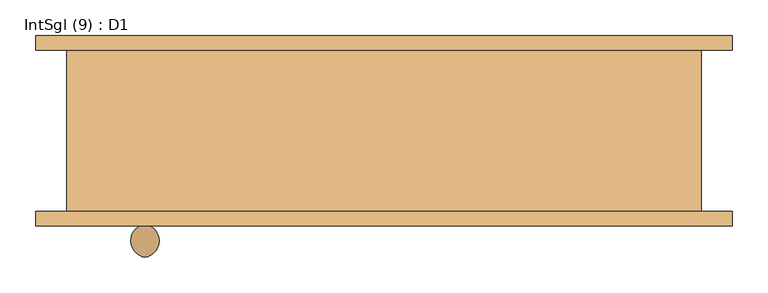
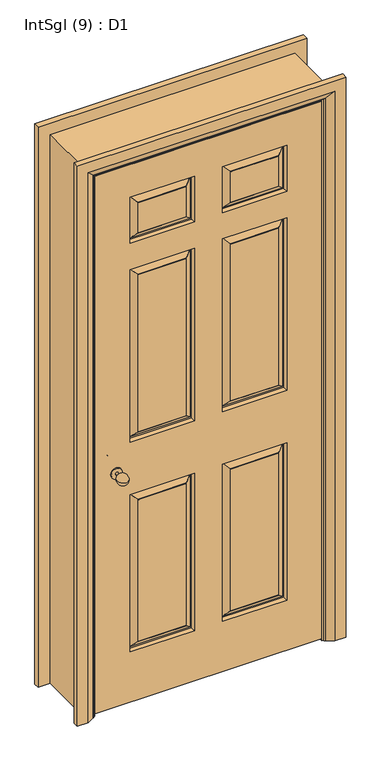
"""IFC4 building model written with IfcOpenShell, lengths in millimetres: door geometry, IntSgl (9) : D1."""

from ifc_helpers import new_model, si_unit, point, frame, origin, place, context, project, spatial, polyline, circle_curve, ellipse_curve, trimmed, outline, extrude, faceted_brep, source, transform, mapped, element, save
from ifc_brep_helpers import plane_surface, cylinder_surface, revolved_surface, advanced_brep


def intsgl_9_d1_bc548916(model_context):
    return source(origin(), model_context, "Body", "SolidModel", [
        advanced_brep(
        [(-328.0, -55.5, 900.0), (-338.0, -55.5, 900.0), (-333.0, -11.062589, 900.0), (-328.0, -70.5, 900.0), (-338.0, -70.5, 900.0), (-353.0, -74.5, 900.0), (-313.0, -74.5, 900.0), (-353.0, -70.5, 900.0), (-313.0, -70.5, 900.0)],
        [
            (0, 1, circle_curve(frame((-333.0, -55.5, 900.0), z_axis=(0.0, 1.0, 0.0), x_axis=(-1.0, 0.0, 0.0)), 5.0)),
            (1, 2, circle_curve(frame((-329.8115138, -33.9213505, 900.0), z_axis=(0.0, 0.0, -1.0), x_axis=(0.0, -1.0, 0.0)), 23.0800654)),
            (2, 0, circle_curve(frame((-336.1884862, -33.9213505, 900.0), z_axis=(0.0, 0.0, -1.0), x_axis=(0.0, -1.0, 0.0)), 23.0800654)),
            (1, 0, circle_curve(frame((-333.0, -55.5, 900.0), z_axis=(0.0, 1.0, 0.0), x_axis=(-1.0, 0.0, 0.0)), 5.0)),
            (0, 3),
            (3, 4, circle_curve(frame((-333.0, -70.5, 900.0), z_axis=(0.0, 1.0, 0.0), x_axis=(-1.0, 0.0, 0.0)), 5.0)),
            (4, 1),
            (4, 3, circle_curve(frame((-333.0, -70.5, 900.0), z_axis=(0.0, 1.0, 0.0), x_axis=(-1.0, 0.0, 0.0)), 5.0)),
            (5, 6, circle_curve(frame((-333.0, -74.5, 900.0), z_axis=(0.0, -1.0, 0.0), x_axis=(1.0, 0.0, 0.0)), 20.0)),
            (6, 5, circle_curve(frame((-333.0, -74.5, 900.0), z_axis=(0.0, -1.0, 0.0), x_axis=(1.0, 0.0, 0.0)), 20.0)),
            (7, 8, circle_curve(frame((-333.0, -70.5, 900.0), z_axis=(0.0, 1.0, 0.0), x_axis=(1.0, 0.0, 0.0)), 20.0)),
            (8, 7, circle_curve(frame((-333.0, -70.5, 900.0), z_axis=(0.0, 1.0, 0.0), x_axis=(1.0, 0.0, 0.0)), 20.0)),
            (5, 7),
            (8, 6),
        ],
        [
            revolved_surface(trimmed(ellipse_curve(frame((-329.8115138, -33.9213505, 900.0), z_axis=(0.0, 0.0, 1.0), x_axis=(0.0, -1.0, 0.0)), 23.0800654, 23.0800654), [point((-333.0, -11.062589, 900.0))], [point((-338.0, -55.5, 900.0))], True, "CARTESIAN"), (-333.0, -70.5, 900.0), (0.0, -1.0, 0.0)),
            cylinder_surface(frame((-333.0, -70.5, 900.0), z_axis=(0.0, -1.0, 0.0), x_axis=(-1.0, 0.0, 0.0)), 5.0),
            plane_surface(frame((-313.0, -74.5, 900.0), z_axis=(0.0, -1.0, 0.0), x_axis=(0.0, 0.0, 1.0))),
            plane_surface(frame((-313.0, -70.5, 900.0), z_axis=(0.0, 1.0, 0.0), x_axis=(0.0, 0.0, -1.0))),
            cylinder_surface(frame((-333.0, -70.5, 900.0), z_axis=(0.0, -1.0, 0.0), x_axis=(1.0, 0.0, 0.0)), 20.0),
        ],
        [
            (0, [[1, 2, 3]]),
            (0, [[-2, 4, -3]]),
            (1, [[-1, 5, 6, 7]]),
            (1, [[-4, -7, 8, -5]]),
            (2, [[9, 10]]),
            (3, [[11, 12], [-6, -8]]),
            (4, [[-9, 13, -12, 14]]),
            (4, [[-10, -14, -11, -13]]),
        ],
    ),
        advanced_brep(
        [(-328.0, -131.5, 900.0), (-333.0, -175.937411, 900.0), (-338.0, -131.5, 900.0), (-338.0, -116.5, 900.0), (-328.0, -116.5, 900.0), (-353.0, -112.5, 900.0), (-313.0, -112.5, 900.0), (-353.0, -116.5, 900.0), (-313.0, -116.5, 900.0)],
        [
            (0, 1, circle_curve(frame((-336.1884862, -153.0786495, 900.0), z_axis=(0.0, 0.0, -1.0), x_axis=(0.0, 1.0, 0.0)), 23.0800654)),
            (1, 2, circle_curve(frame((-329.8115138, -153.0786495, 900.0), z_axis=(0.0, 0.0, -1.0), x_axis=(0.0, 1.0, 0.0)), 23.0800654)),
            (2, 0, circle_curve(frame((-333.0, -131.5, 900.0), z_axis=(0.0, -1.0, 0.0), x_axis=(-1.0, 0.0, 0.0)), 5.0)),
            (0, 2, circle_curve(frame((-333.0, -131.5, 900.0), z_axis=(0.0, -1.0, 0.0), x_axis=(-1.0, 0.0, 0.0)), 5.0)),
            (2, 3),
            (3, 4, circle_curve(frame((-333.0, -116.5, 900.0), z_axis=(0.0, -1.0, 0.0), x_axis=(-1.0, 0.0, 0.0)), 5.0)),
            (4, 0),
            (4, 3, circle_curve(frame((-333.0, -116.5, 900.0), z_axis=(0.0, -1.0, 0.0), x_axis=(-1.0, 0.0, 0.0)), 5.0)),
            (5, 6, circle_curve(frame((-333.0, -112.5, 900.0), z_axis=(0.0, 1.0, 0.0), x_axis=(1.0, 0.0, 0.0)), 20.0)),
            (6, 5, circle_curve(frame((-333.0, -112.5, 900.0), z_axis=(0.0, 1.0, 0.0), x_axis=(1.0, 0.0, 0.0)), 20.0)),
            (7, 8, circle_curve(frame((-333.0, -116.5, 900.0), z_axis=(0.0, -1.0, 0.0), x_axis=(1.0, 0.0, 0.0)), 20.0)),
            (8, 7, circle_curve(frame((-333.0, -116.5, 900.0), z_axis=(0.0, -1.0, 0.0), x_axis=(1.0, 0.0, 0.0)), 20.0)),
            (6, 8),
            (7, 5),
        ],
        [
            revolved_surface(trimmed(ellipse_curve(frame((-329.8115138, -153.0786495, 900.0), z_axis=(0.0, 0.0, -1.0), x_axis=(0.0, 1.0, 0.0)), 23.0800654, 23.0800654), [point((-333.0, -175.937411, 900.0))], [point((-338.0, -131.5, 900.0))], True, "CARTESIAN"), (-333.0, -116.5, 900.0), (0.0, 1.0, 0.0)),
            cylinder_surface(frame((-333.0, -116.5, 900.0), z_axis=(0.0, 1.0, 0.0), x_axis=(-1.0, 0.0, 0.0)), 5.0),
            plane_surface(frame((-313.0, -112.5, 900.0), z_axis=(0.0, 1.0, 0.0), x_axis=(0.0, 0.0, 1.0))),
            plane_surface(frame((-313.0, -116.5, 900.0), z_axis=(0.0, -1.0, 0.0), x_axis=(0.0, 0.0, -1.0))),
            cylinder_surface(frame((-333.0, -116.5, 900.0), z_axis=(0.0, 1.0, 0.0), x_axis=(1.0, 0.0, 0.0)), 20.0),
        ],
        [
            (0, [[1, 2, 3]]),
            (0, [[-1, 4, -2]]),
            (1, [[5, 6, 7, -3]]),
            (1, [[-7, 8, -5, -4]]),
            (2, [[9, 10]]),
            (3, [[11, 12], [-8, -6]]),
            (4, [[13, -11, 14, -10]]),
            (4, [[-14, -12, -13, -9]]),
        ],
    ),
        faceted_brep([(-408.0, -74.5, 2058.0), (408.0, -74.5, 2058.0), (408.0, -74.5, 8.0), (-408.0, -74.5, 8.0), (-50.0, -74.5, 800.0), (-283.0, -74.5, 800.0), (-283.0, -74.5, 200.0), (-50.0, -74.5, 200.0), (283.0, -74.5, 800.0), (50.0, -74.5, 800.0), (50.0, -74.5, 200.0), (283.0, -74.5, 200.0), (-50.0, -74.5, 1658.0), (-283.0, -74.5, 1658.0), (-283.0, -74.5, 1000.0), (-50.0, -74.5, 1000.0), (283.0, -74.5, 1658.0), (50.0, -74.5, 1658.0), (50.0, -74.5, 1000.0), (283.0, -74.5, 1000.0), (-50.0, -74.5, 1933.0), (-283.0, -74.5, 1933.0), (-283.0, -74.5, 1758.0), (-50.0, -74.5, 1758.0), (283.0, -74.5, 1933.0), (50.0, -74.5, 1933.0), (50.0, -74.5, 1758.0), (283.0, -74.5, 1758.0), (-80.0, -74.5, 230.0), (-253.0, -74.5, 230.0), (-253.0, -74.5, 770.0), (-80.0, -74.5, 770.0), (253.0, -74.5, 230.0), (80.0, -74.5, 230.0), (80.0, -74.5, 770.0), (253.0, -74.5, 770.0), (-80.0, -74.5, 1030.0), (-253.0, -74.5, 1030.0), (-253.0, -74.5, 1628.0), (-80.0, -74.5, 1628.0), (253.0, -74.5, 1030.0), (80.0, -74.5, 1030.0), (80.0, -74.5, 1628.0), (253.0, -74.5, 1628.0), (-80.0, -74.5, 1788.0), (-253.0, -74.5, 1788.0), (-253.0, -74.5, 1903.0), (-80.0, -74.5, 1903.0), (253.0, -74.5, 1788.0), (80.0, -74.5, 1788.0), (80.0, -74.5, 1903.0), (253.0, -74.5, 1903.0), (-408.0, -112.5, 2058.0), (-408.0, -112.5, 8.0), (408.0, -112.5, 8.0), (408.0, -112.5, 2058.0), (50.0, -112.5, 800.0), (283.0, -112.5, 800.0), (283.0, -112.5, 200.0), (50.0, -112.5, 200.0), (-283.0, -112.5, 800.0), (-50.0, -112.5, 800.0), (-50.0, -112.5, 200.0), (-283.0, -112.5, 200.0), (50.0, -112.5, 1658.0), (283.0, -112.5, 1658.0), (283.0, -112.5, 1000.0), (50.0, -112.5, 1000.0), (-283.0, -112.5, 1658.0), (-50.0, -112.5, 1658.0), (-50.0, -112.5, 1000.0), (-283.0, -112.5, 1000.0), (50.0, -112.5, 1933.0), (283.0, -112.5, 1933.0), (283.0, -112.5, 1758.0), (50.0, -112.5, 1758.0), (-283.0, -112.5, 1933.0), (-50.0, -112.5, 1933.0), (-50.0, -112.5, 1758.0), (-283.0, -112.5, 1758.0), (80.0, -112.5, 230.0), (253.0, -112.5, 230.0), (253.0, -112.5, 770.0), (80.0, -112.5, 770.0), (-253.0, -112.5, 230.0), (-80.0, -112.5, 230.0), (-80.0, -112.5, 770.0), (-253.0, -112.5, 770.0), (80.0, -112.5, 1030.0), (253.0, -112.5, 1030.0), (253.0, -112.5, 1628.0), (80.0, -112.5, 1628.0), (-253.0, -112.5, 1030.0), (-80.0, -112.5, 1030.0), (-80.0, -112.5, 1628.0), (-253.0, -112.5, 1628.0), (80.0, -112.5, 1788.0), (253.0, -112.5, 1788.0), (253.0, -112.5, 1903.0), (80.0, -112.5, 1903.0), (-253.0, -112.5, 1788.0), (-80.0, -112.5, 1788.0), (-80.0, -112.5, 1903.0), (-253.0, -112.5, 1903.0), (80.0, -111.5, 230.0), (80.0, -111.5, 770.0), (58.0, -97.5, 208.0), (78.0, -111.5, 228.0), (78.0, -111.5, 772.0), (58.0, -97.5, 792.0), (53.0, -97.5, 203.0), (53.0, -97.5, 797.0), (253.0, -111.5, 770.0), (255.0, -111.5, 772.0), (275.0, -97.5, 792.0), (280.0, -97.5, 797.0), (253.0, -111.5, 230.0), (255.0, -111.5, 228.0), (275.0, -97.5, 208.0), (280.0, -97.5, 203.0), (-253.0, -111.5, 230.0), (-253.0, -111.5, 770.0), (-275.0, -97.5, 208.0), (-255.0, -111.5, 228.0), (-255.0, -111.5, 772.0), (-275.0, -97.5, 792.0), (-280.0, -97.5, 203.0), (-280.0, -97.5, 797.0), (-80.0, -111.5, 770.0), (-78.0, -111.5, 772.0), (-58.0, -97.5, 792.0), (-53.0, -97.5, 797.0), (-80.0, -111.5, 230.0), (-78.0, -111.5, 228.0), (-58.0, -97.5, 208.0), (-53.0, -97.5, 203.0), (80.0, -111.5, 1030.0), (80.0, -111.5, 1628.0), (58.0, -97.5, 1008.0), (78.0, -111.5, 1028.0), (78.0, -111.5, 1630.0), (58.0, -97.5, 1650.0), (53.0, -97.5, 1003.0), (53.0, -97.5, 1655.0), (253.0, -111.5, 1628.0), (255.0, -111.5, 1630.0), (275.0, -97.5, 1650.0), (280.0, -97.5, 1655.0), (253.0, -111.5, 1030.0), (255.0, -111.5, 1028.0), (275.0, -97.5, 1008.0), (280.0, -97.5, 1003.0), (-253.0, -111.5, 1030.0), (-253.0, -111.5, 1628.0), (-275.0, -97.5, 1008.0), (-255.0, -111.5, 1028.0), (-255.0, -111.5, 1630.0), (-275.0, -97.5, 1650.0), (-280.0, -97.5, 1003.0), (-280.0, -97.5, 1655.0), (-80.0, -111.5, 1628.0), (-78.0, -111.5, 1630.0), (-58.0, -97.5, 1650.0), (-53.0, -97.5, 1655.0), (-80.0, -111.5, 1030.0), (-78.0, -111.5, 1028.0), (-58.0, -97.5, 1008.0), (-53.0, -97.5, 1003.0), (80.0, -111.5, 1788.0), (80.0, -111.5, 1903.0), (58.0, -97.5, 1766.0), (78.0, -111.5, 1786.0), (78.0, -111.5, 1905.0), (58.0, -97.5, 1925.0), (53.0, -97.5, 1761.0), (53.0, -97.5, 1930.0), (253.0, -111.5, 1903.0), (255.0, -111.5, 1905.0), (275.0, -97.5, 1925.0), (280.0, -97.5, 1930.0), (253.0, -111.5, 1788.0), (255.0, -111.5, 1786.0), (275.0, -97.5, 1766.0), (280.0, -97.5, 1761.0), (-253.0, -111.5, 1788.0), (-253.0, -111.5, 1903.0), (-275.0, -97.5, 1766.0), (-255.0, -111.5, 1786.0), (-255.0, -111.5, 1905.0), (-275.0, -97.5, 1925.0), (-280.0, -97.5, 1761.0), (-280.0, -97.5, 1930.0), (-80.0, -111.5, 1903.0), (-78.0, -111.5, 1905.0), (-58.0, -97.5, 1925.0), (-53.0, -97.5, 1930.0), (-80.0, -111.5, 1788.0), (-78.0, -111.5, 1786.0), (-58.0, -97.5, 1766.0), (-53.0, -97.5, 1761.0), (-80.0, -75.5, 230.0), (-80.0, -75.5, 770.0), (-58.0, -89.5, 208.0), (-78.0, -75.5, 228.0), (-78.0, -75.5, 772.0), (-58.0, -89.5, 792.0), (-53.0, -89.5, 203.0), (-53.0, -89.5, 797.0), (-253.0, -75.5, 770.0), (-255.0, -75.5, 772.0), (-275.0, -89.5, 792.0), (-280.0, -89.5, 797.0), (-253.0, -75.5, 230.0), (-255.0, -75.5, 228.0), (-275.0, -89.5, 208.0), (-280.0, -89.5, 203.0), (253.0, -75.5, 230.0), (253.0, -75.5, 770.0), (275.0, -89.5, 208.0), (255.0, -75.5, 228.0), (255.0, -75.5, 772.0), (275.0, -89.5, 792.0), (280.0, -89.5, 203.0), (280.0, -89.5, 797.0), (80.0, -75.5, 770.0), (78.0, -75.5, 772.0), (58.0, -89.5, 792.0), (53.0, -89.5, 797.0), (80.0, -75.5, 230.0), (78.0, -75.5, 228.0), (58.0, -89.5, 208.0), (53.0, -89.5, 203.0), (-80.0, -75.5, 1030.0), (-80.0, -75.5, 1628.0), (-58.0, -89.5, 1008.0), (-78.0, -75.5, 1028.0), (-78.0, -75.5, 1630.0), (-58.0, -89.5, 1650.0), (-53.0, -89.5, 1003.0), (-53.0, -89.5, 1655.0), (-253.0, -75.5, 1628.0), (-255.0, -75.5, 1630.0), (-275.0, -89.5, 1650.0), (-280.0, -89.5, 1655.0), (-253.0, -75.5, 1030.0), (-255.0, -75.5, 1028.0), (-275.0, -89.5, 1008.0), (-280.0, -89.5, 1003.0), (253.0, -75.5, 1030.0), (253.0, -75.5, 1628.0), (275.0, -89.5, 1008.0), (255.0, -75.5, 1028.0), (255.0, -75.5, 1630.0), (275.0, -89.5, 1650.0), (280.0, -89.5, 1003.0), (280.0, -89.5, 1655.0), (80.0, -75.5, 1628.0), (78.0, -75.5, 1630.0), (58.0, -89.5, 1650.0), (53.0, -89.5, 1655.0), (80.0, -75.5, 1030.0), (78.0, -75.5, 1028.0), (58.0, -89.5, 1008.0), (53.0, -89.5, 1003.0), (-80.0, -75.5, 1788.0), (-80.0, -75.5, 1903.0), (-58.0, -89.5, 1766.0), (-78.0, -75.5, 1786.0), (-78.0, -75.5, 1905.0), (-58.0, -89.5, 1925.0), (-53.0, -89.5, 1761.0), (-53.0, -89.5, 1930.0), (-253.0, -75.5, 1903.0), (-255.0, -75.5, 1905.0), (-275.0, -89.5, 1925.0), (-280.0, -89.5, 1930.0), (-253.0, -75.5, 1788.0), (-255.0, -75.5, 1786.0), (-275.0, -89.5, 1766.0), (-280.0, -89.5, 1761.0), (253.0, -75.5, 1788.0), (253.0, -75.5, 1903.0), (275.0, -89.5, 1766.0), (255.0, -75.5, 1786.0), (255.0, -75.5, 1905.0), (275.0, -89.5, 1925.0), (280.0, -89.5, 1761.0), (280.0, -89.5, 1930.0), (80.0, -75.5, 1903.0), (78.0, -75.5, 1905.0), (58.0, -89.5, 1925.0), (53.0, -89.5, 1930.0), (80.0, -75.5, 1788.0), (78.0, -75.5, 1786.0), (58.0, -89.5, 1766.0), (53.0, -89.5, 1761.0)], [[[0, 1, 2, 3], [4, 5, 6, 7], [8, 9, 10, 11], [12, 13, 14, 15], [16, 17, 18, 19], [20, 21, 22, 23], [24, 25, 26, 27]], [[28, 29, 30, 31]], [[32, 33, 34, 35]], [[36, 37, 38, 39]], [[40, 41, 42, 43]], [[44, 45, 46, 47]], [[48, 49, 50, 51]], [[52, 53, 54, 55], [56, 57, 58, 59], [60, 61, 62, 63], [64, 65, 66, 67], [68, 69, 70, 71], [72, 73, 74, 75], [76, 77, 78, 79]], [[80, 81, 82, 83]], [[84, 85, 86, 87]], [[88, 89, 90, 91]], [[92, 93, 94, 95]], [[96, 97, 98, 99]], [[100, 101, 102, 103]], [[3, 53, 52, 0]], [[2, 54, 53, 3]], [[1, 55, 54, 2]], [[0, 52, 55, 1]], [[104, 80, 83, 105]], [[106, 107, 108, 109]], [[56, 59, 110, 111]], [[83, 82, 112, 105]], [[108, 113, 114, 109]], [[111, 115, 57, 56]], [[82, 81, 116, 112]], [[113, 117, 118, 114]], [[115, 119, 58, 57]], [[104, 116, 81, 80]], [[107, 117, 113, 108], [105, 112, 116, 104]], [[106, 118, 117, 107]], [[110, 119, 115, 111], [109, 114, 118, 106]], [[59, 58, 119, 110]], [[120, 84, 87, 121]], [[122, 123, 124, 125]], [[60, 63, 126, 127]], [[87, 86, 128, 121]], [[124, 129, 130, 125]], [[127, 131, 61, 60]], [[86, 85, 132, 128]], [[129, 133, 134, 130]], [[131, 135, 62, 61]], [[120, 132, 85, 84]], [[123, 133, 129, 124], [121, 128, 132, 120]], [[122, 134, 133, 123]], [[126, 135, 131, 127], [125, 130, 134, 122]], [[63, 62, 135, 126]], [[136, 88, 91, 137]], [[138, 139, 140, 141]], [[64, 67, 142, 143]], [[91, 90, 144, 137]], [[140, 145, 146, 141]], [[143, 147, 65, 64]], [[90, 89, 148, 144]], [[145, 149, 150, 146]], [[147, 151, 66, 65]], [[136, 148, 89, 88]], [[139, 149, 145, 140], [137, 144, 148, 136]], [[138, 150, 149, 139]], [[142, 151, 147, 143], [141, 146, 150, 138]], [[67, 66, 151, 142]], [[152, 92, 95, 153]], [[154, 155, 156, 157]], [[68, 71, 158, 159]], [[95, 94, 160, 153]], [[156, 161, 162, 157]], [[159, 163, 69, 68]], [[94, 93, 164, 160]], [[161, 165, 166, 162]], [[163, 167, 70, 69]], [[152, 164, 93, 92]], [[155, 165, 161, 156], [153, 160, 164, 152]], [[154, 166, 165, 155]], [[158, 167, 163, 159], [157, 162, 166, 154]], [[71, 70, 167, 158]], [[168, 96, 99, 169]], [[170, 171, 172, 173]], [[72, 75, 174, 175]], [[99, 98, 176, 169]], [[172, 177, 178, 173]], [[175, 179, 73, 72]], [[98, 97, 180, 176]], [[177, 181, 182, 178]], [[179, 183, 74, 73]], [[168, 180, 97, 96]], [[171, 181, 177, 172], [169, 176, 180, 168]], [[170, 182, 181, 171]], [[174, 183, 179, 175], [173, 178, 182, 170]], [[75, 74, 183, 174]], [[184, 100, 103, 185]], [[186, 187, 188, 189]], [[76, 79, 190, 191]], [[103, 102, 192, 185]], [[188, 193, 194, 189]], [[191, 195, 77, 76]], [[102, 101, 196, 192]], [[193, 197, 198, 194]], [[195, 199, 78, 77]], [[184, 196, 101, 100]], [[187, 197, 193, 188], [185, 192, 196, 184]], [[186, 198, 197, 187]], [[190, 199, 195, 191], [189, 194, 198, 186]], [[79, 78, 199, 190]], [[200, 28, 31, 201]], [[202, 203, 204, 205]], [[4, 7, 206, 207]], [[31, 30, 208, 201]], [[204, 209, 210, 205]], [[207, 211, 5, 4]], [[30, 29, 212, 208]], [[209, 213, 214, 210]], [[211, 215, 6, 5]], [[200, 212, 29, 28]], [[203, 213, 209, 204], [201, 208, 212, 200]], [[202, 214, 213, 203]], [[206, 215, 211, 207], [205, 210, 214, 202]], [[7, 6, 215, 206]], [[216, 32, 35, 217]], [[218, 219, 220, 221]], [[8, 11, 222, 223]], [[35, 34, 224, 217]], [[220, 225, 226, 221]], [[223, 227, 9, 8]], [[34, 33, 228, 224]], [[225, 229, 230, 226]], [[227, 231, 10, 9]], [[216, 228, 33, 32]], [[219, 229, 225, 220], [217, 224, 228, 216]], [[218, 230, 229, 219]], [[222, 231, 227, 223], [221, 226, 230, 218]], [[11, 10, 231, 222]], [[232, 36, 39, 233]], [[234, 235, 236, 237]], [[12, 15, 238, 239]], [[39, 38, 240, 233]], [[236, 241, 242, 237]], [[239, 243, 13, 12]], [[38, 37, 244, 240]], [[241, 245, 246, 242]], [[243, 247, 14, 13]], [[232, 244, 37, 36]], [[235, 245, 241, 236], [233, 240, 244, 232]], [[234, 246, 245, 235]], [[238, 247, 243, 239], [237, 242, 246, 234]], [[15, 14, 247, 238]], [[248, 40, 43, 249]], [[250, 251, 252, 253]], [[16, 19, 254, 255]], [[43, 42, 256, 249]], [[252, 257, 258, 253]], [[255, 259, 17, 16]], [[42, 41, 260, 256]], [[257, 261, 262, 258]], [[259, 263, 18, 17]], [[248, 260, 41, 40]], [[251, 261, 257, 252], [249, 256, 260, 248]], [[250, 262, 261, 251]], [[254, 263, 259, 255], [253, 258, 262, 250]], [[19, 18, 263, 254]], [[264, 44, 47, 265]], [[266, 267, 268, 269]], [[20, 23, 270, 271]], [[47, 46, 272, 265]], [[268, 273, 274, 269]], [[271, 275, 21, 20]], [[46, 45, 276, 272]], [[273, 277, 278, 274]], [[275, 279, 22, 21]], [[264, 276, 45, 44]], [[267, 277, 273, 268], [265, 272, 276, 264]], [[266, 278, 277, 267]], [[270, 279, 275, 271], [269, 274, 278, 266]], [[23, 22, 279, 270]], [[280, 48, 51, 281]], [[282, 283, 284, 285]], [[24, 27, 286, 287]], [[51, 50, 288, 281]], [[284, 289, 290, 285]], [[287, 291, 25, 24]], [[50, 49, 292, 288]], [[289, 293, 294, 290]], [[291, 295, 26, 25]], [[280, 292, 49, 48]], [[283, 293, 289, 284], [281, 288, 292, 280]], [[282, 294, 293, 283]], [[286, 295, 291, 287], [285, 290, 294, 282]], [[27, 26, 295, 286]]]),
        faceted_brep([(-410.0, -112.5, 0.0), (-442.0, -112.5, 0.0), (-442.0, 112.5, 0.0), (-410.0, 112.5, 0.0), (-410.0, 112.5, 2060.0), (-410.0, -112.5, 2060.0), (-442.0, 112.5, 2092.0), (-442.0, -112.5, 2092.0), (410.0, -112.5, 0.0), (410.0, 112.5, 0.0), (442.0, 112.5, 0.0), (442.0, -112.5, 0.0), (410.0, -112.5, 2060.0), (442.0, -112.5, 2092.0), (442.0, 112.5, 2092.0), (410.0, 112.5, 2060.0)], [[[0, 1, 2, 3]], [[3, 4, 5, 0]], [[2, 6, 4, 3]], [[1, 7, 6, 2]], [[0, 5, 7, 1]], [[8, 9, 10, 11]], [[12, 8, 11, 13]], [[13, 11, 10, 14]], [[14, 10, 9, 15]], [[15, 9, 8, 12]], [[4, 15, 12, 5]], [[6, 14, 15, 4]], [[7, 13, 14, 6]], [[5, 12, 13, 7]]]),
        extrude(outline(polyline([(0.0, -391.0), (2041.0, -391.0), (2041.0, 391.0), (0.0, 391.0), (0.0, 410.0), (2060.0, 410.0), (2060.0, -410.0), (0.0, -410.0), (0.0, -391.0)])), frame((0.0, -72.5, 0.0), z_axis=(0.0, 1.0, 0.0), x_axis=(0.0, 0.0, 1.0)), (0.0, 0.0, 1.0), 32.0),
        advanced_brep(
        [(-485.0, 132.5, 0.0), (-445.0, 132.5, 0.0), (-419.0, 118.5, 0.0), (-415.0, 112.5, 0.0), (-485.0, 112.5, 0.0), (-485.0, 112.5, 2135.0), (-485.0, 132.5, 2135.0), (-415.0, 112.5, 2065.0), (415.0, 112.5, 2065.0), (415.0, 112.5, 0.0), (485.0, 112.5, 0.0), (485.0, 112.5, 2135.0), (-419.0, 118.5, 2069.0), (-445.0, 132.5, 2095.0), (485.0, 132.5, 2135.0), (485.0, 132.5, 0.0), (445.0, 132.5, 0.0), (445.0, 132.5, 2095.0), (419.0, 118.5, 0.0), (419.0, 118.5, 2069.0)],
        [
            (0, 1),
            (1, 2),
            (2, 3, circle_curve(frame((-423.0, 111.5, 0.0), z_axis=(0.0, 0.0, -1.0), x_axis=(-1.0, 0.0, 0.0)), 8.0622577)),
            (3, 4),
            (4, 0),
            (4, 5),
            (5, 6),
            (6, 0),
            (3, 7),
            (7, 8),
            (8, 9),
            (9, 10),
            (10, 11),
            (11, 5),
            (2, 12),
            (12, 7, ellipse_curve(frame((-423.0, 111.5, 2073.0), z_axis=(-0.7071067811865475, 0.0, -0.7071067811865475), x_axis=(0.7071067811865474, 0.0, -0.7071067811865476)), 11.4017543, 8.0622577)),
            (1, 13),
            (13, 12),
            (6, 14),
            (14, 15),
            (15, 16),
            (16, 17),
            (17, 13),
            (10, 15),
            (14, 11),
            (9, 18, circle_curve(frame((423.0, 111.5, 0.0), z_axis=(0.0, 0.0, -1.0), x_axis=(1.0, 0.0, 0.0)), 8.0622577)),
            (18, 16),
            (19, 18),
            (8, 19, ellipse_curve(frame((423.0, 111.5, 2073.0), z_axis=(0.7071067811865475, 0.0, -0.7071067811865475), x_axis=(0.7071067811865474, 0.0, 0.7071067811865476)), 11.4017543, 8.0622577)),
            (19, 17),
            (12, 19),
        ],
        [
            plane_surface(frame((-415.0, 112.5, 0.0), z_axis=(0.0, 0.0, -1.0), x_axis=(0.0, 1.0, 0.0))),
            plane_surface(frame((-485.0, 132.5, 0.0), z_axis=(-1.0, 0.0, 0.0), x_axis=(0.0, 0.0, 1.0))),
            plane_surface(frame((-485.0, 112.5, 0.0), z_axis=(0.0, -1.0, 0.0), x_axis=(0.0, 0.0, 1.0))),
            cylinder_surface(frame((-423.0, 111.5, 0.0), z_axis=(0.0, 0.0, -1.0), x_axis=(-1.0, 0.0, 0.0)), 8.0622577),
            plane_surface(frame((-419.0, 118.5, 0.0), z_axis=(0.4740998230350183, 0.8804710999221749, 0.0), x_axis=(0.0, 0.0, 1.0))),
            plane_surface(frame((-445.0, 132.5, 0.0), z_axis=(0.0, 1.0, 0.0), x_axis=(0.0, 0.0, 1.0))),
            plane_surface(frame((485.0, 132.5, 2135.0), z_axis=(1.0, 0.0, 0.0), x_axis=(0.0, 0.0, -1.0))),
            plane_surface(frame((415.0, 112.5, 0.0), z_axis=(0.0, 0.0, -1.0), x_axis=(0.0, 1.0, 0.0))),
            cylinder_surface(frame((423.0, 111.5, 2065.0), z_axis=(0.0, 0.0, 1.0), x_axis=(1.0, 0.0, 0.0)), 8.0622577),
            plane_surface(frame((419.0, 118.5, 2069.0), z_axis=(-0.4740998230350183, 0.8804710999221749, 0.0), x_axis=(0.0, 0.0, -1.0))),
            plane_surface(frame((-485.0, 132.5, 2135.0), z_axis=(0.0, 0.0, 1.0), x_axis=(1.0, 0.0, 0.0))),
            cylinder_surface(frame((-415.0, 111.5, 2073.0), z_axis=(-1.0, 0.0, 0.0), x_axis=(0.0, 0.0, 1.0)), 8.0622577),
            plane_surface(frame((-419.0, 118.5, 2069.0), z_axis=(0.0, 0.8804710999221749, -0.4740998230350183), x_axis=(1.0, 0.0, 0.0))),
        ],
        [
            (0, [[1, 2, 3, 4, 5]]),
            (1, [[6, 7, 8, -5]]),
            (2, [[9, 10, 11, 12, 13, 14, -6, -4]]),
            (3, [[15, 16, -9, -3]]),
            (4, [[17, 18, -15, -2]]),
            (5, [[-8, 19, 20, 21, 22, 23, -17, -1]]),
            (6, [[-13, 24, -20, 25]]),
            (7, [[-24, -12, 26, 27, -21]]),
            (8, [[28, -26, -11, 29]]),
            (9, [[-22, -27, -28, 30]]),
            (10, [[-14, -25, -19, -7]]),
            (11, [[31, -29, -10, -16]]),
            (12, [[-23, -30, -31, -18]]),
        ],
    ),
        advanced_brep(
        [(485.0, -132.5, 0.0), (445.0, -132.5, 0.0), (419.0, -118.5, 0.0), (415.0, -112.5, 0.0), (485.0, -112.5, 0.0), (485.0, -112.5, 2135.0), (485.0, -132.5, 2135.0), (415.0, -112.5, 2065.0), (-415.0, -112.5, 2065.0), (-415.0, -112.5, 0.0), (-485.0, -112.5, 0.0), (-485.0, -112.5, 2135.0), (419.0, -118.5, 2069.0), (445.0, -132.5, 2095.0), (-485.0, -132.5, 2135.0), (-485.0, -132.5, 0.0), (-445.0, -132.5, 0.0), (-445.0, -132.5, 2095.0), (-419.0, -118.5, 0.0), (-419.0, -118.5, 2069.0)],
        [
            (0, 1),
            (1, 2),
            (2, 3, circle_curve(frame((423.0, -111.5, 0.0), z_axis=(0.0, 0.0, -1.0), x_axis=(1.0, 0.0, 0.0)), 8.0622577)),
            (3, 4),
            (4, 0),
            (4, 5),
            (5, 6),
            (6, 0),
            (3, 7),
            (7, 8),
            (8, 9),
            (9, 10),
            (10, 11),
            (11, 5),
            (2, 12),
            (12, 7, ellipse_curve(frame((423.0, -111.5, 2073.0), z_axis=(0.7071067811865475, 0.0, -0.7071067811865475), x_axis=(-0.7071067811865474, 0.0, -0.7071067811865476)), 11.4017543, 8.0622577)),
            (1, 13),
            (13, 12),
            (6, 14),
            (14, 15),
            (15, 16),
            (16, 17),
            (17, 13),
            (10, 15),
            (14, 11),
            (9, 18, circle_curve(frame((-423.0, -111.5, 0.0), z_axis=(0.0, 0.0, -1.0), x_axis=(-1.0, 0.0, 0.0)), 8.0622577)),
            (18, 16),
            (19, 18),
            (8, 19, ellipse_curve(frame((-423.0, -111.5, 2073.0), z_axis=(-0.7071067811865475, 0.0, -0.7071067811865475), x_axis=(-0.7071067811865474, 0.0, 0.7071067811865476)), 11.4017543, 8.0622577)),
            (19, 17),
            (12, 19),
        ],
        [
            plane_surface(frame((415.0, -112.5, 0.0), z_axis=(0.0, 0.0, -1.0), x_axis=(0.0, -1.0, 0.0))),
            plane_surface(frame((485.0, -132.5, 0.0), z_axis=(1.0, 0.0, 0.0), x_axis=(0.0, 0.0, 1.0))),
            plane_surface(frame((485.0, -112.5, 0.0), z_axis=(0.0, 1.0, 0.0), x_axis=(0.0, 0.0, 1.0))),
            cylinder_surface(frame((423.0, -111.5, 0.0), z_axis=(0.0, 0.0, -1.0), x_axis=(1.0, 0.0, 0.0)), 8.0622577),
            plane_surface(frame((419.0, -118.5, 0.0), z_axis=(-0.4740998230350183, -0.8804710999221749, 0.0), x_axis=(0.0, 0.0, 1.0))),
            plane_surface(frame((445.0, -132.5, 0.0), z_axis=(0.0, -1.0, 0.0), x_axis=(0.0, 0.0, 1.0))),
            plane_surface(frame((-485.0, -132.5, 2135.0), z_axis=(-1.0, 0.0, 0.0), x_axis=(0.0, 0.0, -1.0))),
            plane_surface(frame((-415.0, -112.5, 0.0), z_axis=(0.0, 0.0, -1.0), x_axis=(0.0, -1.0, 0.0))),
            cylinder_surface(frame((-423.0, -111.5, 2065.0), z_axis=(0.0, 0.0, 1.0), x_axis=(-1.0, 0.0, 0.0)), 8.0622577),
            plane_surface(frame((-419.0, -118.5, 2069.0), z_axis=(0.4740998230350183, -0.8804710999221749, 0.0), x_axis=(0.0, 0.0, -1.0))),
            plane_surface(frame((485.0, -132.5, 2135.0), z_axis=(0.0, 0.0, 1.0), x_axis=(-1.0, 0.0, 0.0))),
            cylinder_surface(frame((415.0, -111.5, 2073.0), z_axis=(1.0, 0.0, 0.0), x_axis=(0.0, 0.0, 1.0)), 8.0622577),
            plane_surface(frame((419.0, -118.5, 2069.0), z_axis=(0.0, -0.8804710999221749, -0.4740998230350183), x_axis=(-1.0, 0.0, 0.0))),
        ],
        [
            (0, [[1, 2, 3, 4, 5]]),
            (1, [[6, 7, 8, -5]]),
            (2, [[9, 10, 11, 12, 13, 14, -6, -4]]),
            (3, [[15, 16, -9, -3]]),
            (4, [[17, 18, -15, -2]]),
            (5, [[-8, 19, 20, 21, 22, 23, -17, -1]]),
            (6, [[-13, 24, -20, 25]]),
            (7, [[-24, -12, 26, 27, -21]]),
            (8, [[28, -26, -11, 29]]),
            (9, [[-22, -27, -28, 30]]),
            (10, [[-14, -25, -19, -7]]),
            (11, [[31, -29, -10, -16]]),
            (12, [[-23, -30, -31, -18]]),
        ],
    ),
    ])


if __name__ == "__main__":
    model = new_model("IFC4")
    model_context = context("Model", 3, world=origin())
    ifc_project = project(units=[si_unit("LENGTHUNIT", "METRE", prefix="MILLI")], contexts=[model_context])
    site = spatial("IfcSite", under=ifc_project)
    building = spatial("IfcBuilding", under=site)
    placement = place(None, origin())
    intsgl_9_d1_shape = intsgl_9_d1_bc548916(model_context)
    element("IfcDoor", 1, ObjectType="IntSgl (9) : D1", at=placement, inside=building, context=model_context, shape_type="MappedRepresentation", body=[
        mapped(intsgl_9_d1_shape, transform((0.0, 0.0, 0.0), x_axis=(1.0, 0.0, 0.0), y_axis=(0.0, 1.0, 0.0), z_axis=(0.0, 0.0, 1.0))),
    ])
    save(model, "model.ifc")

# Revit data of these elements
# Type "IntSgl (9) : D1"
#   Type Mark = "46"
#   Operation = "SingleSwingRight"
#   Manufacturer = "Revit"
#   Keynote = "L20"
#   UnderCut = 8 mm
#   Tolerance = 2 mm
#   Thickness = 38 mm
#   Structural Tolerance = 8 mm
#   StopDepth = 32 mm
#   Stop Thickness = 19 mm
#   Stile Top Rail = 125 mm
#   Stile Shutting = 125 mm
#   Stile Muntin Rail = 100 mm
#   Stile Lock Rail = 200 mm
#   Stile Intermediate/Frieze = 100 mm
#   Stile Hanging = 125 mm
#   Stile Bottom Rail = 200 mm
#   Rough Width = 900 mm
#   Rough Height = 2100 mm
#   Height to Top Lock Rail = 1000 mm
#   Handle Z Distance = 900 mm
#   Handle X Distance = 75 mm
#   Frame Thickness = 32 mm
#   Door Panel Width = 816 mm
#   Height = 2100 mm
#   Width = 900 mm
#   Door Panel Thickness = 38 mm
#   Door Panel Offset = 0 mm
#   Door Panel Height = 2050 mm
#   Architrave Setback = 5 mm
#   Vis - Ironmongery = yes
#   Material Ironmongery = Door - Handle
#   Material Frame = Door - Frame/Mullion
#   Material Door = Door - Panel
#   Material Architrave = Door - Architrave
#   Function = (empty or 0)
#   Wall Closure = (empty or 0)
# Element 1 (IfcDoor, "IntSgl (9) : D1")
#   Materials on its faces: "Door - Panel", "Door - Architrave", "Door - Frame/Mullion", "Door - Handle"
# Materials
#   "Door - Handle": colour RGB 247 247 247, transparency 0
#   "Door - Frame/Mullion": colour RGB 212 179 113, transparency 0
#   "Door - Panel": colour RGB 154 90 5, transparency 0
#   "Door - Architrave": colour RGB 154 90 5, transparency 0
